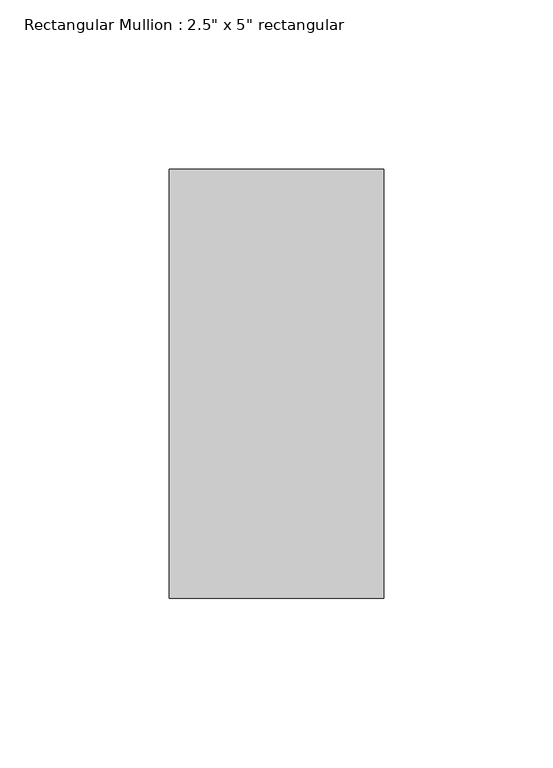
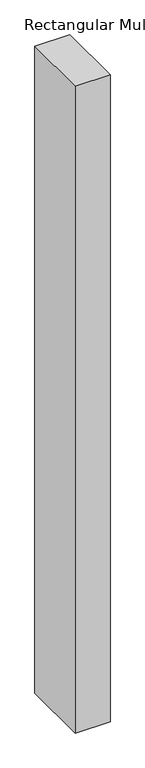
"""IFC4 building model written with IfcOpenShell, lengths in millimetres: member geometry."""

from ifc_helpers import new_model, si_unit, frame, origin, place, context, project, spatial, polyline, outline, extrude, source, transform, mapped, element, save


def member_a1da5be3(model_context):
    return source(origin(), model_context, "Body", "SweptSolid", [
        extrude(outline(polyline([(31.75, 63.5), (31.75, -63.5), (-31.75, -63.5), (-31.75, 63.5), (31.75, 63.5)])), frame((0.0, 0.0, -1244.6), z_axis=(0.0, 0.0, 1.0), x_axis=(1.0, 0.0, 0.0)), (0.0, 0.0, 1.0), 1244.6),
    ])


if __name__ == "__main__":
    model = new_model("IFC4")
    model_context = context("Model", 3, world=origin())
    ifc_project = project(units=[si_unit("LENGTHUNIT", "METRE", prefix="MILLI")], contexts=[model_context])
    site = spatial("IfcSite", under=ifc_project)
    building = spatial("IfcBuilding", under=site)
    placement = place(None, origin())
    member_shape = member_a1da5be3(model_context)
    element("IfcMember", 1, ObjectType="Rectangular Mullion : 2.5\" x 5\" rectangular", at=placement, inside=building, context=model_context, shape_type="MappedRepresentation", body=[
        mapped(member_shape, transform((0.0, 0.0, 0.0), x_axis=(1.0, 0.0, 0.0), y_axis=(0.0, 1.0, 0.0), z_axis=(0.0, 0.0, 1.0))),
    ])
    save(model, "model.ifc")

# Revit data of these elements
# Type "Rectangular Mullion : 2.5\" x 5\" rectangular"
#   built-in parameter 1007304 = 0.416667 (stored number, unit not read)
#   built-in parameter 1007301 = 0.104167 (stored number, unit not read)
#   built-in parameter 1007300 = 0.104167 (stored number, unit not read)
# Element 1 (IfcMember, "Rectangular Mullion : 2.5\" x 5\" rectangular")
#   Materials on its faces: "WINDOW FRAMING"
# Materials
#   "WINDOW FRAMING": class "Generic", colour RGB 120 120 120, transparency 0, Cost = 0
